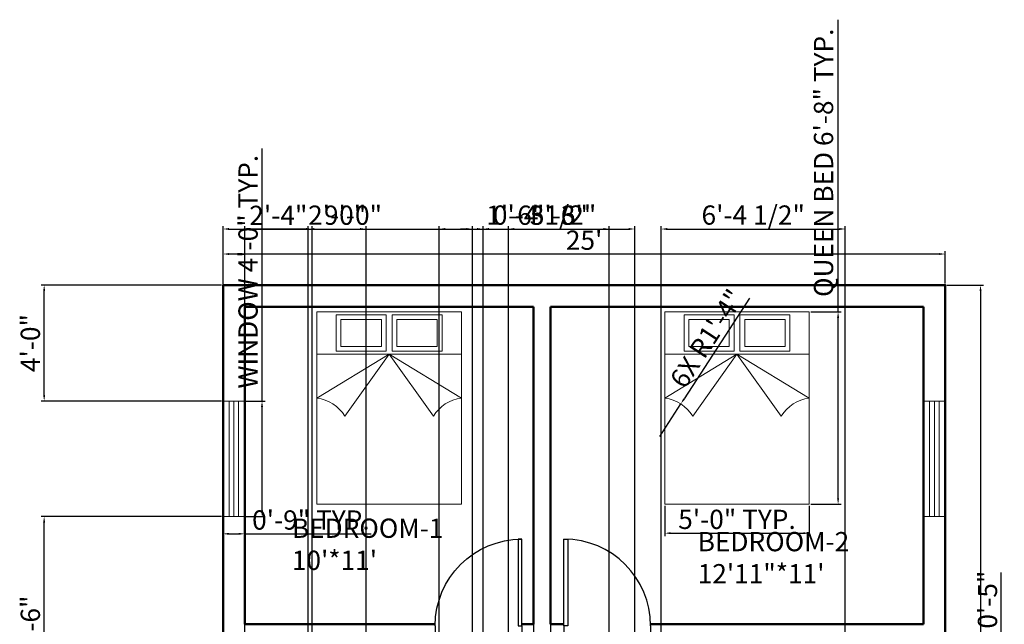
# Model space of a CAD drawing. Units: inches. Extents: x 2528 to 2954, y 1660 to 2209.
# Tile 4 of 4: x 2534 to 2943, y 1957 to 2209. Entities that reach past the tile are written whole.
import ezdxf

# ---------------------------------------------------------------- set-up
doc = ezdxf.new("R2010")
doc.units = ezdxf.units.IN
for name, color, linetype, lineweight in [('A-ANNO-DIMS', 5, 'Continuous', 18), ('A-AREA-IDEN', 5, 'Continuous', 25), ('DOOR', 3, 'Continuous', 25), ('FURNITURE', 6, 'Continuous', 18), ('WALL', 1, 'Continuous', 50), ('WINDOW', 4, 'Continuous', 18)]:
    doc.layers.add(name, color=color, linetype=linetype, lineweight=lineweight)
doc.styles.get("Standard").update_dxf_attribs({"font": 'arial.ttf'})
doc.dimstyles.new('ISO-25', dxfattribs={"dimtxt": 8, "dimasz": 2.5, "dimexe": 1.25, "dimexo": 0.625, "dimtad": 1, "dimlunit": 3, "dimtxsty": 'Standard', "dimcen": 2.5, "dimadec": 0, "dimazin": 0, "dimtfac": 1, "dimtmove": 0, "dimatfit": 3, "dimfxl": 1, "dimarcsym": 0})

# ---------------------------------------------------------------- blocks, each defined once
blk = doc.blocks.new('*U2')
for p, q in [((0, 0), (0, -6)), ((40, 0), (40, -6))]:
    blk.add_line(p, q)
blk.add_lwpolyline([(0, 0), (0, 40), (1.75, 40), (1.75, 0)], close=True)
blk.add_arc((0, 0), 40, 0, 90)
blk = doc.blocks.new('*D11')
at = {"layer": 'A-ANNO-DIMS', "color": 0, "lineweight": -2, "transparency": 16777216}
for p, q in [((2618.92, 2099.01), (2618.92, 2112.55)), ((2916.42, 2111.3), (2621.42, 2111.3)), ((2918.92, 2099.01), (2918.92, 2112.55))]:
    blk.add_line(p, q, dxfattribs=at)
at = {"layer": 'A-ANNO-DIMS', "color": 0, "transparency": 16777216}
for points in [[(2621.42, 2111.71), (2621.42, 2110.88), (2618.92, 2111.3)], [(2916.42, 2111.71), (2916.42, 2110.88), (2918.92, 2111.3)]]:
    blk.add_solid(points, dxfattribs=at)
at = {"layer": 'Defpoints', "color": 0, "transparency": 16777216}
for p in [(2618.92, 2111.3), (2618.92, 2098.39), (2918.92, 2098.39)]:
    blk.add_point(p, dxfattribs=at)
at = {"layer": 'A-ANNO-DIMS', "color": 0, "transparency": 16777216, "insert": (2768.92, 2116.01), "char_height": 8, "attachment_point": 5}
blk.add_mtext("25'", dxfattribs=at)
blk = doc.blocks.new('*D12')
at = {"layer": 'A-ANNO-DIMS', "color": 0, "lineweight": -2, "transparency": 16777216}
for p, q in [((2919.54, 2098.39), (2934.84, 2098.39)), ((2933.59, 2095.89), (2933.59, 1716.89)), ((2919.54, 1714.39), (2934.84, 1714.39))]:
    blk.add_line(p, q, dxfattribs=at)
at = {"layer": 'A-ANNO-DIMS', "color": 0, "transparency": 16777216}
for points in [[(2933.17, 2095.89), (2934.01, 2095.89), (2933.59, 2098.39)], [(2933.17, 1716.89), (2934.01, 1716.89), (2933.59, 1714.39)]]:
    blk.add_solid(points, dxfattribs=at)
at = {"layer": 'Defpoints', "color": 0, "transparency": 16777216}
for p in [(2918.92, 2098.39), (2918.92, 1714.39), (2933.59, 1714.39)]:
    blk.add_point(p, dxfattribs=at)
at = {"layer": 'A-ANNO-DIMS', "color": 0, "transparency": 16777216, "insert": (2928.88, 1906.39), "char_height": 8, "attachment_point": 5, "rotation": 90}
blk.add_mtext("32'", dxfattribs=at)
blk = doc.blocks.new('BED-QUEEN-60X80')
for p, q in [((0, 0), (0, 80)), ((0, 80), (60, 80)), ((8, 78.8), (28.8, 78.8)), ((8, 65.6), (8, 78.8)), ((28.8, 78.8), (28.8, 63.6)), ((31.2, 78.8), (52, 78.8)), ((31.2, 65.6), (31.2, 78.8)), ((52, 78.8), (52, 63.6)), ((60, 80), (60, 0)), ((10, 76.8), (26.8, 76.8)), ((10, 65.6), (10, 76.8)), ((26.8, 76.8), (26.8, 65.6)), ((33.2, 65.6), (33.2, 76.8)), ((33.2, 76.8), (50, 76.8)), ((50, 76.8), (50, 65.6)), ((8, 63.6), (8, 65.6)), ((26.8, 65.6), (10, 65.6)), ((31.2, 63.6), (31.2, 65.6)), ((50, 65.6), (33.2, 65.6)), ((60, 62.4), (0, 62.4)), ((30, 62.4), (0, 44.18)), ((28.8, 63.6), (8, 63.6)), ((11.62, 36.62), (30, 62.4)), ((30, 62.4), (60, 44.18)), ((48.38, 36.62), (30, 62.4)), ((52, 63.6), (31.2, 63.6)), ((52, 62.4), (31.2, 62.4)), ((60, 0), (0, 0))]:
    blk.add_line(p, q)
for centre, start, end in [((-2.1, 28.24), 31.4416, 82.4986), ((62.1, 28.24), 97.5014, 148.5584)]:
    blk.add_arc(centre, 16.08, start, end)
blk = doc.blocks.new('WIN-48IN')
for p, q in [((0, 48), (9, 48)), ((2.5, 0), (2.5, 48)), ((4.5, 0), (4.5, 48)), ((6.5, 0), (6.5, 48)), ((9, 0), (0, 0))]:
    blk.add_line(p, q)
blk = doc.blocks.new('*D17')
at = {"layer": 'A-ANNO-DIMS', "color": 0, "lineweight": -2, "transparency": 16777216}
for p, q in [((2635.12, 2050.2), (2635.12, 2155.18)), ((2628.54, 2050.2), (2636.37, 2050.2)), ((2635.12, 2004.7), (2635.12, 2047.7)), ((2628.54, 2002.2), (2636.37, 2002.2))]:
    blk.add_line(p, q, dxfattribs=at)
at = {"layer": 'A-ANNO-DIMS', "color": 0, "transparency": 16777216}
for points in [[(2634.7, 2047.7), (2635.53, 2047.7), (2635.12, 2050.2)], [(2634.7, 2004.7), (2635.53, 2004.7), (2635.12, 2002.2)]]:
    blk.add_solid(points, dxfattribs=at)
at = {"layer": 'Defpoints', "color": 0, "transparency": 16777216}
for p in [(2627.92, 2050.2), (2635.12, 2050.2), (2627.92, 2002.2)]:
    blk.add_point(p, dxfattribs=at)
at = {"layer": 'A-ANNO-DIMS', "color": 0, "transparency": 16777216, "insert": (2630.35, 2103.94), "char_height": 8, "attachment_point": 5, "rotation": 90}
blk.add_mtext('WINDOW 4\'-0" TYP.', dxfattribs=at)
blk = doc.blocks.new('*D18')
at = {"layer": 'A-ANNO-DIMS', "color": 0, "lineweight": -2, "transparency": 16777216}
for p, q in [((2618.92, 2001.57), (2618.92, 1993.75)), ((2627.92, 2001.57), (2627.92, 1993.75)), ((2621.42, 1995), (2625.42, 1995)), ((2627.92, 1995), (2680.43, 1995))]:
    blk.add_line(p, q, dxfattribs=at)
at = {"layer": 'A-ANNO-DIMS', "color": 0, "transparency": 16777216}
for points in [[(2621.42, 1995.41), (2621.42, 1994.58), (2618.92, 1995)], [(2625.42, 1995.41), (2625.42, 1994.58), (2627.92, 1995)]]:
    blk.add_solid(points, dxfattribs=at)
at = {"layer": 'Defpoints', "color": 0, "transparency": 16777216}
for p in [(2618.92, 2002.2), (2627.92, 2002.2), (2627.92, 1995)]:
    blk.add_point(p, dxfattribs=at)
at = {"layer": 'A-ANNO-DIMS', "color": 0, "transparency": 16777216, "insert": (2655.42, 1999.71), "char_height": 8, "attachment_point": 5}
blk.add_mtext('0\'-9" TYP.', dxfattribs=at)
blk = doc.blocks.new('*D21')
at = {"layer": 'A-ANNO-DIMS', "color": 0, "lineweight": -2, "transparency": 16777216}
for p, q in [((2874.42, 2087.27), (2874.42, 2208.7)), ((2863.04, 2087.27), (2875.67, 2087.27)), ((2874.42, 2009.77), (2874.42, 2084.77)), ((2863.04, 2007.27), (2875.67, 2007.27))]:
    blk.add_line(p, q, dxfattribs=at)
at = {"layer": 'A-ANNO-DIMS', "color": 0, "transparency": 16777216}
for points in [[(2874, 2084.77), (2874.83, 2084.77), (2874.42, 2087.27)], [(2874, 2009.77), (2874.83, 2009.77), (2874.42, 2007.27)]]:
    blk.add_solid(points, dxfattribs=at)
at = {"layer": 'Defpoints', "color": 0, "transparency": 16777216}
for p in [(2862.42, 2087.27), (2874.42, 2087.27), (2862.42, 2007.27)]:
    blk.add_point(p, dxfattribs=at)
at = {"layer": 'A-ANNO-DIMS', "color": 0, "transparency": 16777216, "insert": (2869.41, 2149.23), "char_height": 8, "attachment_point": 5, "rotation": 90}
blk.add_mtext('QUEEN BED 6\'-8" TYP.', dxfattribs=at)
blk = doc.blocks.new('*D22')
at = {"layer": 'A-ANNO-DIMS', "color": 0, "lineweight": -2, "transparency": 16777216}
for p, q in [((2802.42, 2006.64), (2802.42, 1994.02)), ((2862.42, 2006.64), (2862.42, 1994.02)), ((2804.92, 1995.27), (2859.92, 1995.27))]:
    blk.add_line(p, q, dxfattribs=at)
at = {"layer": 'A-ANNO-DIMS', "color": 0, "transparency": 16777216}
for points in [[(2804.92, 1995.69), (2804.92, 1994.85), (2802.42, 1995.27)], [(2859.92, 1995.69), (2859.92, 1994.85), (2862.42, 1995.27)]]:
    blk.add_solid(points, dxfattribs=at)
at = {"layer": 'Defpoints', "color": 0, "transparency": 16777216}
for p in [(2802.42, 2007.27), (2862.42, 2007.27), (2862.42, 1995.27)]:
    blk.add_point(p, dxfattribs=at)
at = {"layer": 'A-ANNO-DIMS', "color": 0, "transparency": 16777216, "insert": (2832.42, 1999.98), "char_height": 8, "attachment_point": 5}
blk.add_mtext('5\'-0" TYP.', dxfattribs=at)
blk = doc.blocks.new('*D30')
at = {"layer": 'A-ANNO-DIMS', "color": 0, "lineweight": -2, "transparency": 16777216}
for p, q in [((2618.29, 2002.2), (2543.37, 2002.2)), ((2544.62, 1914.89), (2544.62, 1999.7)), ((2618.29, 1912.39), (2543.37, 1912.39))]:
    blk.add_line(p, q, dxfattribs=at)
at = {"layer": 'A-ANNO-DIMS', "color": 0, "transparency": 16777216}
for points in [[(2544.2, 1999.7), (2545.03, 1999.7), (2544.62, 2002.2)], [(2544.2, 1914.89), (2545.03, 1914.89), (2544.62, 1912.39)]]:
    blk.add_solid(points, dxfattribs=at)
at = {"layer": 'Defpoints', "color": 0, "transparency": 16777216}
for p in [(2544.62, 2002.2), (2618.92, 2002.2), (2618.92, 1912.39)]:
    blk.add_point(p, dxfattribs=at)
at = {"layer": 'A-ANNO-DIMS', "color": 0, "transparency": 16777216, "insert": (2539.91, 1957.29), "char_height": 8, "attachment_point": 5, "rotation": 90}
blk.add_mtext('7\'-6"', dxfattribs=at)
blk = doc.blocks.new('*D31')
at = {"layer": 'A-ANNO-DIMS', "color": 0, "lineweight": -2, "transparency": 16777216}
for p, q in [((2618.29, 2098.39), (2543.37, 2098.39)), ((2544.62, 2052.7), (2544.62, 2095.89)), ((2618.29, 2050.2), (2543.37, 2050.2))]:
    blk.add_line(p, q, dxfattribs=at)
at = {"layer": 'A-ANNO-DIMS', "color": 0, "transparency": 16777216}
for points in [[(2544.2, 2095.89), (2545.03, 2095.89), (2544.62, 2098.39)], [(2544.2, 2052.7), (2545.03, 2052.7), (2544.62, 2050.2)]]:
    blk.add_solid(points, dxfattribs=at)
at = {"layer": 'Defpoints', "color": 0, "transparency": 16777216}
for p in [(2544.62, 2098.39), (2618.92, 2098.39), (2618.92, 2050.2)]:
    blk.add_point(p, dxfattribs=at)
at = {"layer": 'A-ANNO-DIMS', "color": 0, "transparency": 16777216, "insert": (2539.91, 2074.29), "char_height": 8, "attachment_point": 5, "rotation": 90}
blk.add_mtext('4\'-0"', dxfattribs=at)
blk = doc.blocks.new('*D34')
at = {"layer": 'A-ANNO-DIMS', "color": 0, "lineweight": -2, "transparency": 16777216}
for p, q in [((2618.92, 1715.01), (2618.92, 2122.94)), ((2726.92, 1703.01), (2726.92, 2122.94)), ((2621.42, 2121.69), (2724.42, 2121.69))]:
    blk.add_line(p, q, dxfattribs=at)
at = {"layer": 'A-ANNO-DIMS', "color": 0, "transparency": 16777216}
for points in [[(2621.42, 2122.11), (2621.42, 2121.27), (2618.92, 2121.69)], [(2724.42, 2122.11), (2724.42, 2121.27), (2726.92, 2121.69)]]:
    blk.add_solid(points, dxfattribs=at)
at = {"layer": 'Defpoints', "color": 0, "transparency": 16777216}
for p in [(2726.92, 2121.69), (2618.92, 1714.39), (2726.92, 1702.39)]:
    blk.add_point(p, dxfattribs=at)
at = {"layer": 'A-ANNO-DIMS', "color": 0, "transparency": 16777216, "insert": (2672.92, 2126.4), "char_height": 8, "attachment_point": 5}
blk.add_mtext('9\'-0"', dxfattribs=at)
blk = doc.blocks.new('*D35')
at = {"layer": 'A-ANNO-DIMS', "color": 0, "lineweight": -2, "transparency": 16777216}
for p, q in [((2726.92, 1691.01), (2726.92, 2122.94)), ((2789.92, 1691.01), (2789.92, 2122.94)), ((2729.42, 2121.69), (2787.42, 2121.69))]:
    blk.add_line(p, q, dxfattribs=at)
at = {"layer": 'A-ANNO-DIMS', "color": 0, "transparency": 16777216}
for points in [[(2729.42, 2122.11), (2729.42, 2121.27), (2726.92, 2121.69)], [(2787.42, 2122.11), (2787.42, 2121.27), (2789.92, 2121.69)]]:
    blk.add_solid(points, dxfattribs=at)
at = {"layer": 'Defpoints', "color": 0, "transparency": 16777216}
for p in [(2789.92, 2121.69), (2726.92, 1690.39), (2789.92, 1690.39)]:
    blk.add_point(p, dxfattribs=at)
at = {"layer": 'A-ANNO-DIMS', "color": 0, "transparency": 16777216, "insert": (2758.42, 2126.4), "char_height": 8, "attachment_point": 5}
blk.add_mtext('5\'-3"', dxfattribs=at)
blk = doc.blocks.new('*D37')
at = {"layer": 'A-ANNO-DIMS', "color": 0, "lineweight": -2, "transparency": 16777216}
for p, q in [((2737.46, 1724.01), (2737.46, 2122.94)), ((2779.37, 1724.01), (2779.37, 2122.94)), ((2739.96, 2121.69), (2776.87, 2121.69))]:
    blk.add_line(p, q, dxfattribs=at)
at = {"layer": 'A-ANNO-DIMS', "color": 0, "transparency": 16777216}
for points in [[(2739.96, 2122.11), (2739.96, 2121.27), (2737.46, 2121.69)], [(2776.87, 2122.11), (2776.87, 2121.27), (2779.37, 2121.69)]]:
    blk.add_solid(points, dxfattribs=at)
at = {"layer": 'Defpoints', "color": 0, "transparency": 16777216}
for p in [(2779.37, 2121.69), (2737.46, 1723.39), (2779.37, 1723.39)]:
    blk.add_point(p, dxfattribs=at)
at = {"layer": 'A-ANNO-DIMS', "color": 0, "transparency": 16777216, "insert": (2758.42, 2126.4), "char_height": 8, "attachment_point": 5}
blk.add_mtext('3\'-6"', dxfattribs=at)
blk = doc.blocks.new('*D39')
at = {"layer": 'A-ANNO-DIMS', "color": 0, "lineweight": -2, "transparency": 16777216}
for p, q in [((2654.34, 1947.01), (2654.34, 2122.94)), ((2678.32, 1947.01), (2678.32, 2122.94)), ((2656.84, 2121.69), (2675.82, 2121.69))]:
    blk.add_line(p, q, dxfattribs=at)
at = {"layer": 'A-ANNO-DIMS', "color": 0, "transparency": 16777216}
for points in [[(2656.84, 2122.11), (2656.84, 2121.27), (2654.34, 2121.69)], [(2675.82, 2122.11), (2675.82, 2121.27), (2678.32, 2121.69)]]:
    blk.add_solid(points, dxfattribs=at)
at = {"layer": 'Defpoints', "color": 0, "transparency": 16777216}
for p in [(2678.32, 2121.69), (2654.34, 1946.38), (2678.32, 1946.38)]:
    blk.add_point(p, dxfattribs=at)
at = {"layer": 'A-ANNO-DIMS', "color": 0, "transparency": 16777216, "insert": (2666.33, 2126.4), "char_height": 8, "attachment_point": 5}
blk.add_mtext('2\'-0"', dxfattribs=at)
blk = doc.blocks.new('*D41')
at = {"layer": 'A-ANNO-DIMS', "color": 0, "lineweight": -2, "transparency": 16777216}
for p, q in [((2800.92, 1952.01), (2800.92, 2122.94)), ((2877.42, 1952.01), (2877.42, 2122.94)), ((2803.42, 2121.69), (2874.92, 2121.69))]:
    blk.add_line(p, q, dxfattribs=at)
at = {"layer": 'A-ANNO-DIMS', "color": 0, "transparency": 16777216}
for points in [[(2803.42, 2122.11), (2803.42, 2121.27), (2800.92, 2121.69)], [(2874.92, 2122.11), (2874.92, 2121.27), (2877.42, 2121.69)]]:
    blk.add_solid(points, dxfattribs=at)
at = {"layer": 'Defpoints', "color": 0, "transparency": 16777216}
for p in [(2877.42, 2121.69), (2800.92, 1951.39), (2877.42, 1951.39)]:
    blk.add_point(p, dxfattribs=at)
at = {"layer": 'A-ANNO-DIMS', "color": 0, "transparency": 16777216, "insert": (2839.17, 2126.45), "char_height": 8, "attachment_point": 5}
blk.add_mtext('6\'-4 1/2"', dxfattribs=at)
blk = doc.blocks.new('*D45')
at = {"layer": 'A-ANNO-DIMS', "color": 0, "lineweight": -2, "transparency": 16777216}
for p, q in [((2708.76, 1744.99), (2708.76, 2122.94)), ((2726.92, 1748.01), (2726.92, 2122.94)), ((2711.26, 2121.69), (2724.42, 2121.69)), ((2726.92, 2121.69), (2751.18, 2121.69))]:
    blk.add_line(p, q, dxfattribs=at)
at = {"layer": 'A-ANNO-DIMS', "color": 0, "transparency": 16777216}
for points in [[(2711.26, 2122.11), (2711.26, 2121.27), (2708.76, 2121.69)], [(2724.42, 2122.11), (2724.42, 2121.27), (2726.92, 2121.69)]]:
    blk.add_solid(points, dxfattribs=at)
at = {"layer": 'Defpoints', "color": 0, "transparency": 16777216}
for p in [(2726.92, 2121.69), (2726.92, 1747.39), (2708.76, 1744.37)]:
    blk.add_point(p, dxfattribs=at)
at = {"layer": 'A-ANNO-DIMS', "color": 0, "transparency": 16777216, "insert": (2740.3, 2126.4), "char_height": 8, "attachment_point": 5}
blk.add_mtext('1\'-6"', dxfattribs=at)
blk = doc.blocks.new('*D47')
at = {"layer": 'A-ANNO-DIMS', "color": 0, "lineweight": -2, "transparency": 16777216}
for p, q in [((2627.92, 1913.01), (2627.92, 2122.94)), ((2655.91, 1902.51), (2655.91, 2122.94)), ((2653.41, 2121.69), (2630.42, 2121.69))]:
    blk.add_line(p, q, dxfattribs=at)
at = {"layer": 'A-ANNO-DIMS', "color": 0, "transparency": 16777216}
for points in [[(2630.42, 2122.11), (2630.42, 2121.27), (2627.92, 2121.69)], [(2653.41, 2122.11), (2653.41, 2121.27), (2655.91, 2121.69)]]:
    blk.add_solid(points, dxfattribs=at)
at = {"layer": 'Defpoints', "color": 0, "transparency": 16777216}
for p in [(2627.92, 2121.69), (2627.92, 1912.39), (2655.91, 1901.89)]:
    blk.add_point(p, dxfattribs=at)
at = {"layer": 'A-ANNO-DIMS', "color": 0, "transparency": 16777216, "insert": (2641.91, 2126.33), "char_height": 8, "attachment_point": 5}
blk.add_mtext('2\'-4"', dxfattribs=at)
blk = doc.blocks.new('*D48')
at = {"layer": 'A-ANNO-DIMS', "color": 0, "lineweight": -2, "transparency": 16777216}
for p, q in [((2747.92, 2088.76), (2747.92, 1665.84)), ((2754.92, 2088.76), (2754.92, 1665.84)), ((2750.42, 1667.09), (2752.42, 1667.09)), ((2754.92, 1667.09), (2779.93, 1667.09))]:
    blk.add_line(p, q, dxfattribs=at)
at = {"layer": 'A-ANNO-DIMS', "color": 0, "transparency": 16777216}
for points in [[(2750.42, 1667.51), (2750.42, 1666.67), (2747.92, 1667.09)], [(2752.42, 1667.51), (2752.42, 1666.67), (2754.92, 1667.09)]]:
    blk.add_solid(points, dxfattribs=at)
at = {"layer": 'Defpoints', "color": 0, "transparency": 16777216}
for p in [(2747.92, 2089.39), (2754.92, 2089.39), (2754.92, 1667.09)]:
    blk.add_point(p, dxfattribs=at)
at = {"layer": 'A-ANNO-DIMS', "color": 0, "transparency": 16777216, "insert": (2768.67, 1671.8), "char_height": 8, "attachment_point": 5}
blk.add_mtext('0\'-7"', dxfattribs=at)
blk = doc.blocks.new('*D52')
at = {"layer": 'A-ANNO-DIMS', "color": 0, "lineweight": -2, "transparency": 16777216}
for p, q in [((2942.22, 1953.89), (2942.22, 1978.91)), ((2676.54, 1951.39), (2943.47, 1951.39)), ((2942.22, 1946.38), (2942.22, 1951.39)), ((2682.54, 1946.38), (2943.47, 1946.38)), ((2942.22, 1943.88), (2942.22, 1941.38))]:
    blk.add_line(p, q, dxfattribs=at)
at = {"layer": 'A-ANNO-DIMS', "color": 0, "transparency": 16777216}
for points in [[(2941.8, 1953.89), (2942.63, 1953.89), (2942.22, 1951.39)], [(2941.8, 1943.88), (2942.63, 1943.88), (2942.22, 1946.38)]]:
    blk.add_solid(points, dxfattribs=at)
at = {"layer": 'Defpoints', "color": 0, "transparency": 16777216}
for p in [(2675.92, 1951.39), (2942.22, 1951.39), (2681.92, 1946.38)]:
    blk.add_point(p, dxfattribs=at)
at = {"layer": 'A-ANNO-DIMS', "color": 0, "transparency": 16777216, "insert": (2937.51, 1967.65), "char_height": 8, "attachment_point": 5, "rotation": 90}
blk.add_mtext('0\'-5"', dxfattribs=at)
blk = doc.blocks.new('*D54')
at = {"layer": 'A-ANNO-DIMS', "color": 0, "lineweight": -2, "transparency": 16777216}
for p, q in [((2722.51, 1827.01), (2722.51, 2122.94)), ((2726.92, 1827.01), (2726.92, 2122.94)), ((2720.01, 2121.69), (2717.51, 2121.69)), ((2722.51, 2121.69), (2726.92, 2121.69)), ((2729.42, 2121.69), (2773.07, 2121.69))]:
    blk.add_line(p, q, dxfattribs=at)
at = {"layer": 'A-ANNO-DIMS', "color": 0, "transparency": 16777216}
for points in [[(2720.01, 2122.11), (2720.01, 2121.27), (2722.51, 2121.69)], [(2729.42, 2122.11), (2729.42, 2121.27), (2726.92, 2121.69)]]:
    blk.add_solid(points, dxfattribs=at)
at = {"layer": 'Defpoints', "color": 0, "transparency": 16777216}
for p in [(2726.92, 2121.69), (2722.51, 1826.39), (2726.92, 1826.39)]:
    blk.add_point(p, dxfattribs=at)
at = {"layer": 'A-ANNO-DIMS', "color": 0, "transparency": 16777216, "insert": (2752.49, 2126.45), "char_height": 8, "attachment_point": 5}
blk.add_mtext('0\'-4 1/2"', dxfattribs=at)
blk = doc.blocks.new('*D58')
at = {"layer": 'A-ANNO-DIMS', "color": 0, "lineweight": -2, "transparency": 16777216}
for p, q in [((2837.65, 2092.92), (2810.44, 2051.08)), ((2800.32, 2035.51), (2809.08, 2048.99))]:
    blk.add_line(p, q, dxfattribs=at)
at = {"layer": 'A-ANNO-DIMS', "color": 0, "transparency": 16777216}
blk.add_solid([(2810.09, 2051.31), (2810.79, 2050.85), (2809.08, 2048.99)], dxfattribs=at)
at = {"layer": 'Defpoints', "color": 0, "transparency": 16777216}
for p in [(2809.08, 2048.99), (2800.32, 2035.51)]:
    blk.add_point(p, dxfattribs=at)
at = {"layer": 'A-ANNO-DIMS', "color": 0, "transparency": 16777216, "insert": (2820.78, 2075.62), "char_height": 8, "attachment_point": 5, "rotation": 56.9697}
blk.add_mtext('6X R1\'-4"', dxfattribs=at)

msp = doc.modelspace()

# ---------------------------------------------------------------- linework, layer by layer
at = {"layer": 'WALL'}
for p, q in [((2627.915, 2089.389), (2747.915, 2089.389)), ((2627.915, 1957.389), (2627.915, 2089.389)), ((2747.915, 1957.389), (2747.915, 2089.389)), ((2754.915, 2089.389), (2754.915, 1957.389)), ((2754.915, 2089.389), (2909.915, 2089.389)), ((2909.915, 2089.389), (2909.915, 1957.389)), ((2627.915, 1957.389), (2707.053, 1957.389)), ((2743.048, 1957.389), (2747.915, 1957.389)), ((2754.915, 1957.389), (2760.539, 1957.389)), ((2909.915, 1957.389), (2796.539, 1957.389))]:
    msp.add_line(p, q, dxfattribs=at)
msp.add_lwpolyline([(2618.915, 2098.389), (2918.915, 2098.389), (2918.915, 1714.389), (2618.915, 1714.389)], close=True, dxfattribs=at)

# ---------------------------------------------------------------- block references
at = {"layer": 'DOOR', "yscale": 0.9, "zscale": 0.9}
for p, xscale in [((2743.048, 1956.789), -0.9), ((2760.539, 1956.789), 0.9)]:
    msp.add_blockref('*U2', p, dxfattribs=dict(at, xscale=xscale))
at = {"layer": 'FURNITURE'}
for p in [(2657.915, 2007.269), (2802.415, 2007.269)]:
    msp.add_blockref('BED-QUEEN-60X80', p, dxfattribs=at)
at = {"layer": 'WINDOW'}
msp.add_blockref('WIN-48IN', (2618.915, 2002.198), dxfattribs=at)
at = {"layer": 'WINDOW', "rotation": 180}
msp.add_blockref('WIN-48IN', (2918.915, 2050.197), dxfattribs=at)

# ---------------------------------------------------------------- texts
at = {"layer": 'A-AREA-IDEN', "char_height": 8, "attachment_point": 1}
for s, width, insert in [("BEDROOM-1\\P10'*11'", 135.45159, (2647.514, 2001.331)), ('BEDROOM-2\\P12\'11"*11\'', 35.96736, (2816.094, 1995.756))]:
    msp.add_mtext_dynamic_manual_height_columns(s, width=width, gutter_width=12.5, heights=[0], dxfattribs=dict(at, insert=insert))

# ---------------------------------------------------------------- dimensions: what is measured, and where the dimension line sits
at = {"layer": 'A-ANNO-DIMS'}
for base, p1, p2, text, picture, middle in [((2874.415, 2087.269), (2862.415, 2007.269), (2862.415, 2087.269), 'QUEEN BED <> TYP.', '*D21', (2869.408, 2149.235)), ((2635.115, 2050.198), (2627.915, 2002.198), (2627.915, 2050.198), 'WINDOW <> TYP.', '*D17', (2630.351, 2103.939))]:
    dim = msp.add_linear_dim(base=base, p1=p1, p2=p2, angle=90, text=text, dimstyle='ISO-25', override={"dimdec": 1, "dimlfac": 1, "dimrnd": 0, "dimzin": 1, "dimdsep": 46, "dimlunit": 4, "dimfrac": 2}, dxfattribs=at)
    dim.commit()
    dim.dimension.update_dxf_attribs({"geometry": picture, "text_midpoint": middle})
for base, p1, p2, override, picture, middle in [((2726.915, 2121.689), (2722.508, 1826.389), (2726.915, 1826.389), {"dimdec": 1, "dimlfac": 1, "dimrnd": 0, "dimzin": 1, "dimdsep": 46, "dimlunit": 4, "dimfrac": 2}, '*D54', (2752.494, 2126.451)), ((2877.423, 2121.689), (2800.915, 1951.389), (2877.423, 1951.389), {"dimdec": 1, "dimlfac": 1, "dimrnd": 0, "dimzin": 1, "dimdsep": 46, "dimlunit": 4, "dimfrac": 2}, '*D41', (2839.169, 2126.451)), ((2726.915, 2121.689), (2618.915, 1714.389), (2726.915, 1702.389), {"dimdec": 1, "dimlfac": 1, "dimrnd": 0, "dimzin": 1, "dimdsep": 46, "dimlunit": 4, "dimfrac": 2}, '*D34', (2672.915, 2126.399)), ((2627.915, 2121.689), (2655.915, 1901.889), (2627.915, 1912.389), {"dimdec": 1, "dimlfac": 1, "dimrnd": 0, "dimzin": 1, "dimdsep": 46, "dimlunit": 4, "dimfrac": 2}, '*D47', (2641.915, 2126.331)), ((2678.318, 2121.689), (2654.338, 1946.385), (2678.318, 1946.385), {"dimdec": 1, "dimlfac": 1, "dimrnd": 0, "dimzin": 1, "dimdsep": 46, "dimlunit": 4, "dimfrac": 2}, '*D39', (2666.328, 2126.399)), ((2726.915, 2121.689), (2708.757, 1744.369), (2726.915, 1747.389), {"dimdec": 1, "dimlfac": 1, "dimrnd": 0, "dimzin": 1, "dimdsep": 46, "dimlunit": 4, "dimfrac": 2}, '*D45', (2740.296, 2126.399)), ((2789.915, 2121.689), (2726.915, 1690.389), (2789.915, 1690.389), {"dimdec": 1, "dimlfac": 1, "dimrnd": 0, "dimzin": 1, "dimdsep": 46, "dimlunit": 4, "dimfrac": 2}, '*D35', (2758.415, 2126.402)), ((2779.374, 2121.689), (2737.461, 1723.389), (2779.374, 1723.389), {"dimdec": 1, "dimlfac": 1, "dimrnd": 0, "dimzin": 1, "dimdsep": 46, "dimlunit": 4, "dimfrac": 2}, '*D37', (2758.418, 2126.402)), ((2618.915, 2111.296), (2918.915, 2098.389), (2618.915, 2098.389), {"dimclrd": 0, "dimclre": 0, "dimclrt": 0}, '*D11', (2768.915, 2116.006)), ((2754.915, 1667.089), (2747.915, 2089.389), (2754.915, 2089.389), {"dimdec": 1, "dimlfac": 1, "dimrnd": 0, "dimzin": 1, "dimdsep": 46, "dimlunit": 4, "dimfrac": 2}, '*D48', (2768.673, 1671.799))]:
    dim = msp.add_linear_dim(base=base, p1=p1, p2=p2, dimstyle='ISO-25', override=override, dxfattribs=at)
    dim.commit()
    dim.dimension.update_dxf_attribs({"geometry": picture, "text_midpoint": middle})
for base, p1, p2, override, picture, middle in [((2544.615, 2098.389), (2618.915, 2050.198), (2618.915, 2098.389), {"dimdec": 1, "dimlfac": 1, "dimrnd": 0, "dimzin": 1, "dimdsep": 46, "dimlunit": 4, "dimfrac": 2}, '*D31', (2539.905, 2074.293)), ((2933.588, 1714.389), (2918.915, 2098.389), (2918.915, 1714.389), {"dimclrd": 0, "dimclre": 0, "dimclrt": 0}, '*D12', (2928.876, 1906.389)), ((2544.615, 2002.198), (2618.915, 1912.389), (2618.915, 2002.198), {"dimdec": 1, "dimlfac": 1, "dimrnd": 0, "dimzin": 1, "dimdsep": 46, "dimlunit": 4, "dimfrac": 2}, '*D30', (2539.905, 1957.293)), ((2942.215, 1951.389), (2681.915, 1946.385), (2675.915, 1951.389), {"dimdec": 1, "dimlfac": 1, "dimrnd": 0, "dimzin": 1, "dimdsep": 46, "dimlunit": 4, "dimfrac": 2}, '*D52', (2937.505, 1967.647))]:
    dim = msp.add_linear_dim(base=base, p1=p1, p2=p2, angle=90, dimstyle='ISO-25', override=override, dxfattribs=at)
    dim.commit()
    dim.dimension.update_dxf_attribs({"geometry": picture, "text_midpoint": middle})
dim = msp.add_radius_dim(center=(2800.316, 2035.505), mpoint=(2809.08, 2048.985), text='6X <>', dimstyle='ISO-25', override={"dimdec": 1, "dimlfac": 1, "dimrnd": 0, "dimzin": 1, "dimdsep": 46, "dimlunit": 4, "dimfrac": 2}, dxfattribs=at)
dim.commit()
dim.dimension.update_dxf_attribs({"geometry": '*D58', "text_midpoint": (2820.777, 2075.616)})
for base, p1, p2, picture, middle in [((2627.915, 1994.998), (2618.915, 2002.198), (2627.915, 2002.198), '*D18', (2655.422, 1999.707)), ((2862.415, 1995.269), (2802.415, 2007.269), (2862.415, 2007.269), '*D22', (2832.415, 1999.979))]:
    dim = msp.add_linear_dim(base=base, p1=p1, p2=p2, text='<> TYP.', dimstyle='ISO-25', override={"dimdec": 1, "dimlfac": 1, "dimrnd": 0, "dimzin": 1, "dimdsep": 46, "dimlunit": 4, "dimfrac": 2}, dxfattribs=at)
    dim.commit()
    dim.dimension.update_dxf_attribs({"geometry": picture, "text_midpoint": middle})

doc.saveas('drawing.dxf')
